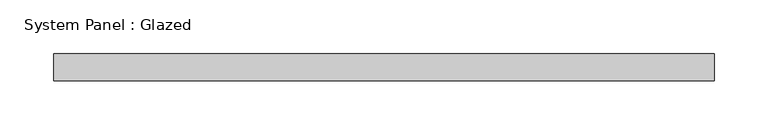
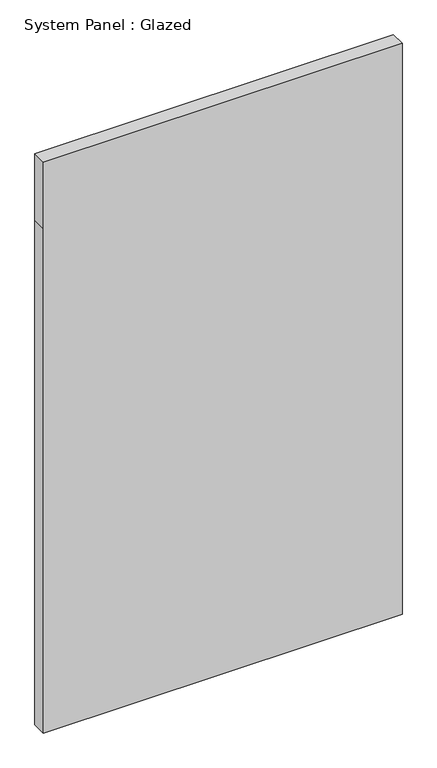
"""IFC4 building model written with IfcOpenShell, lengths in millimetres: plate geometry, System Panel : Glazed."""

from ifc_helpers import new_model, si_unit, frame, origin, place, context, project, spatial, polyline, outline, extrude, source, transform, mapped, element, save


def system_panel_glazed_8182dcf9(model_context):
    return source(origin(), model_context, "Body", "SweptSolid", [
        extrude(outline(polyline([(0.0, -307.975), (0.0, 307.975), (916.2309713, 307.975), (1036.8809713, 307.975), (1036.8809713, -307.975), (916.2309713, -307.975), (0.0, -307.975)])), frame((0.0, 19.05, 0.0), z_axis=(0.0, 1.0, 0.0), x_axis=(0.0, 0.0, 1.0)), (0.0, 0.0, 1.0), 25.4),
    ])


if __name__ == "__main__":
    model = new_model("IFC4")
    model_context = context("Model", 3, world=origin())
    ifc_project = project(units=[si_unit("LENGTHUNIT", "METRE", prefix="MILLI")], contexts=[model_context])
    site = spatial("IfcSite", under=ifc_project)
    building = spatial("IfcBuilding", under=site)
    placement = place(None, origin())
    system_panel_glazed_shape = system_panel_glazed_8182dcf9(model_context)
    element("IfcPlate", 1, ObjectType="System Panel : Glazed", at=placement, inside=building, context=model_context, shape_type="MappedRepresentation", body=[
        mapped(system_panel_glazed_shape, transform((0.0, 0.0, 0.0), x_axis=(1.0, 0.0, 0.0), y_axis=(0.0, 1.0, 0.0), z_axis=(0.0, 0.0, 1.0))),
    ])
    save(model, "model.ifc")

# Revit data of these elements
# Type "System Panel : Glazed"
#   Construction Type Id = "GSP4R"
#   Analytic Construction = "1/8 in Pilkington single glazing"
#   Visual Light Transmittance = 0.9
#   Solar Heat Gain Coefficient = 0.86
#   Heat Transfer Coefficient (U) = 1.18115 BTU/(h·ft²·°F)
#   Define Thermal Properties by = 1
# Element 1 (IfcPlate, "System Panel : Glazed")
#   Materials on its faces: "Glass"
# Materials
#   "Glass": class "Glass", colour RGB 0 128 192, transparency 0.75, Description = "Soda Lime Glass", Cost = 0
